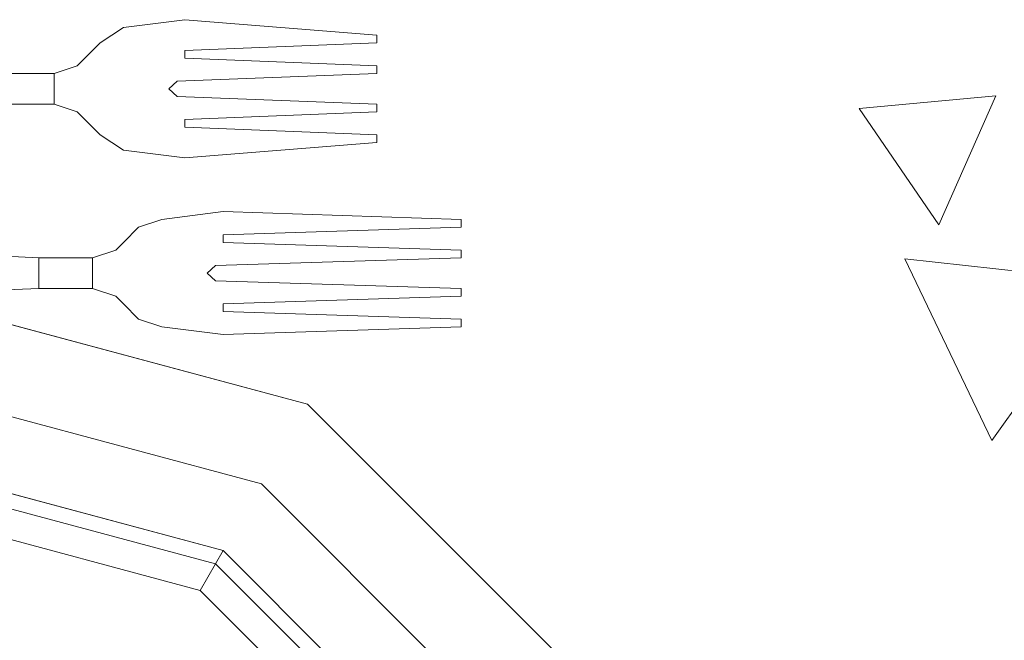
# Model space of a CAD drawing. Units: inches. Extents: x 375 to 1122, y 27 to 1069.
# Tile 103 of 155: x 713.015 to 720.91, y 872.174 to 877.148. Entities that reach past the tile are written whole.
import ezdxf

# ---------------------------------------------------------------- set-up
doc = ezdxf.new("R2010")
doc.units = ezdxf.units.IN
doc.layers.add('Furniture', color=30, linetype='Continuous', lineweight=18)

# ---------------------------------------------------------------- blocks, each defined once
blk = doc.blocks.new('A$C403C54AD')
for p, q in [((1.57741, 0.87913, -0.0006), (1.58183, 0.91926, -0.0006)), ((1.58183, 0.91926, -0.0006), (1.61385, 0.89659, -0.0006)), ((1.54732, 0.87, -0.0006), (1.54475, 0.89734, -0.0006)), ((1.54475, 0.89734, -0.0006), (1.57064, 0.88596, -0.0006)), ((1.61385, 0.89659, -0.0006), (1.57741, 0.87913, -0.0006)), ((1.57064, 0.88596, -0.0006), (1.54732, 0.87, -0.0006)), ((1.56951, 0.73013, -0.02105), (1.57105, 0.72551, -0.02059)), ((1.56951, 0.73013, -0.02413), (1.57105, 0.72551, -0.02367)), ((1.53103, 0.72244, -0.02105), (1.53411, 0.71782, -0.02059)), ((1.53103, 0.72244, -0.02413), (1.53411, 0.71782, -0.02367))]:
    blk.add_line(p, q)
at = {"linetype": 'ByBlock'}
for points, invisible_edges in [([(1.65725, 0.81008, -0.00874), (1.66648, 0.79408, -0.00874), (1.62254, 0.75014, -0.00874), (1.60654, 0.75938, -0.00874)], 5), ([(1.67418, 0.78075, -0.02259), (1.65725, 0.81008, -0.01335), (1.60654, 0.75938, -0.01335), (1.63587, 0.74244, -0.02259)], 5), ([(1.66648, 0.79408, -0.00874), (1.67572, 0.77809, -0.01489), (1.63853, 0.74091, -0.01489), (1.62254, 0.75014, -0.00874)], 5), ([(1.6788, 0.77276, -0.03183), (1.67418, 0.78075, -0.02259), (1.63587, 0.74244, -0.02259), (1.64387, 0.73783, -0.03183)], 1), ([(1.67572, 0.77809, -0.01489), (1.72651, 0.69011, -0.01489), (1.72651, 0.69011, -0.01489), (1.63853, 0.74091, -0.01489)], 5), ([(1.60654, 0.75938, -0.00874), (1.62254, 0.75014, -0.00874), (1.60645, 0.69011, -0.00874), (1.58798, 0.69011, -0.00874)], 5), ([(1.63587, 0.74244, -0.02259), (1.60654, 0.75938, -0.01335), (1.58798, 0.69011, -0.01335), (1.62185, 0.69011, -0.02259)], 5), ([(1.62254, 0.75014, -0.00874), (1.63853, 0.74091, -0.01489), (1.62492, 0.69011, -0.01489), (1.60645, 0.69011, -0.00874)], 5), ([(1.63853, 0.74091, -0.01489), (1.72651, 0.69011, -0.01489), (1.72651, 0.69011, -0.01489), (1.62492, 0.69011, -0.01489)], 5)]:
    blk.add_3dface(points, dxfattribs=dict(at, invisible_edges=invisible_edges))
for points in [[(1.65725, 0.81008, -0.01335), (1.65725, 0.81008, -0.00874), (1.60654, 0.75938, -0.00874), (1.60654, 0.75938, -0.01335)], [(1.60654, 0.75938, -0.01335), (1.60654, 0.75938, -0.00874), (1.58798, 0.69011, -0.00874), (1.58798, 0.69011, -0.01335)], [(1.64387, 0.73783, -0.03183), (1.63587, 0.74244, -0.02259), (1.62185, 0.69011, -0.02259), (1.63108, 0.69011, -0.03183)]]:
    blk.add_3dface(points, dxfattribs=at)
for points, invisible_edges in [([(1.57259, 0.74244, -0.02045), (1.56797, 0.74244, -0.02045), (1.56951, 0.79016, -0.01335), (1.57105, 0.79016, -0.01335)], 1), ([(1.57259, 0.74244, -0.02353), (1.56797, 0.74244, -0.02353), (1.56951, 0.79016, -0.01643), (1.57105, 0.79016, -0.01643)], 1), ([(1.57875, 0.74091, -0.0207), (1.57413, 0.74244, -0.02045), (1.57567, 0.79016, -0.01335), (1.57721, 0.79016, -0.01335)], 1), ([(1.57875, 0.74091, -0.02378), (1.57413, 0.74244, -0.02353), (1.57567, 0.79016, -0.01643), (1.57721, 0.79016, -0.01643)], 1), ([(1.58645, 0.74244, -0.02045), (1.58183, 0.74091, -0.0207), (1.58337, 0.79016, -0.01335), (1.58491, 0.79016, -0.01335)], 1), ([(1.58645, 0.74244, -0.02353), (1.58183, 0.74091, -0.02378), (1.58337, 0.79016, -0.01643), (1.58491, 0.79016, -0.01643)], 1), ([(1.58798, 0.74244, -0.02045), (1.5926, 0.74244, -0.02045), (1.59106, 0.79016, -0.01335), (1.58952, 0.79016, -0.01335)], 1), ([(1.58798, 0.74244, -0.02353), (1.5926, 0.74244, -0.02353), (1.59106, 0.79016, -0.01643), (1.58952, 0.79016, -0.01643)], 1), ([(1.53565, 0.73475, -0.02045), (1.5295, 0.73475, -0.02045), (1.53257, 0.77323, -0.01335), (1.53411, 0.77323, -0.01335)], 1), ([(1.53565, 0.73475, -0.02353), (1.5295, 0.73475, -0.02353), (1.53257, 0.77323, -0.01643), (1.53411, 0.77323, -0.01643)], 1), ([(1.54181, 0.73321, -0.0207), (1.53719, 0.73475, -0.02045), (1.53873, 0.77323, -0.01335), (1.54027, 0.77323, -0.01335)], 1), ([(1.54181, 0.73321, -0.02378), (1.53719, 0.73475, -0.02353), (1.53873, 0.77323, -0.01643), (1.54027, 0.77323, -0.01643)], 1), ([(1.5495, 0.73475, -0.02045), (1.54489, 0.73321, -0.0207), (1.54643, 0.77323, -0.01335), (1.54797, 0.77323, -0.01335)], 1), ([(1.5495, 0.73475, -0.02353), (1.54489, 0.73321, -0.02378), (1.54643, 0.77323, -0.01643), (1.54797, 0.77323, -0.01643)], 1), ([(1.55104, 0.73475, -0.02045), (1.5572, 0.73475, -0.02045), (1.55412, 0.77323, -0.01335), (1.55258, 0.77323, -0.01335)], 1), ([(1.55104, 0.73475, -0.02353), (1.5572, 0.73475, -0.02353), (1.55412, 0.77323, -0.01643), (1.55258, 0.77323, -0.01643)], 1), ([(1.56951, 0.73013, -0.02105), (1.57413, 0.74244, -0.02045), (1.57259, 0.74244, -0.02045), (1.56797, 0.74244, -0.02045)], 5), ([(1.56951, 0.73013, -0.02413), (1.57413, 0.74244, -0.02353), (1.57259, 0.74244, -0.02353), (1.56797, 0.74244, -0.02353)], 5), ([(1.56951, 0.73013, -0.02413), (1.56951, 0.73013, -0.02105), (1.56797, 0.74244, -0.02045), (1.56797, 0.74244, -0.02353)], 1), ([(1.56951, 0.73013, -0.02105), (1.58029, 0.73924, -0.02085), (1.57875, 0.74091, -0.0207), (1.57413, 0.74244, -0.02045)], 13), ([(1.56951, 0.73013, -0.02413), (1.58029, 0.73924, -0.02392), (1.57875, 0.74091, -0.02378), (1.57413, 0.74244, -0.02353)], 13), ([(1.59106, 0.73013, -0.02105), (1.58029, 0.73924, -0.02085), (1.58183, 0.74091, -0.0207), (1.58645, 0.74244, -0.02045)], 13), ([(1.59106, 0.73013, -0.02413), (1.58029, 0.73924, -0.02392), (1.58183, 0.74091, -0.02378), (1.58645, 0.74244, -0.02353)], 13), ([(1.59106, 0.73013, -0.02105), (1.58645, 0.74244, -0.02045), (1.58798, 0.74244, -0.02045), (1.5926, 0.74244, -0.02045)], 5), ([(1.59106, 0.73013, -0.02413), (1.58645, 0.74244, -0.02353), (1.58798, 0.74244, -0.02353), (1.5926, 0.74244, -0.02353)], 5), ([(1.59106, 0.73013, -0.02105), (1.59106, 0.73013, -0.02413), (1.5926, 0.74244, -0.02353), (1.5926, 0.74244, -0.02045)], 1), ([(1.59106, 0.73013, -0.02105), (1.58029, 0.73924, -0.02085), (1.56951, 0.73013, -0.02105), (1.59106, 0.73013, -0.02105)], 7), ([(1.59106, 0.73013, -0.02413), (1.58029, 0.73924, -0.02392), (1.56951, 0.73013, -0.02413), (1.59106, 0.73013, -0.02413)], 7), ([(1.53103, 0.72244, -0.02105), (1.53719, 0.73475, -0.02045), (1.53565, 0.73475, -0.02045), (1.5295, 0.73475, -0.02045)], 5), ([(1.53103, 0.72244, -0.02413), (1.53719, 0.73475, -0.02353), (1.53565, 0.73475, -0.02353), (1.5295, 0.73475, -0.02353)], 5), ([(1.53103, 0.72244, -0.02413), (1.53103, 0.72244, -0.02105), (1.5295, 0.73475, -0.02045), (1.5295, 0.73475, -0.02353)], 1), ([(1.53103, 0.72244, -0.02105), (1.54335, 0.73155, -0.02085), (1.54181, 0.73321, -0.0207), (1.53719, 0.73475, -0.02045)], 13), ([(1.53103, 0.72244, -0.02413), (1.54335, 0.73155, -0.02392), (1.54181, 0.73321, -0.02378), (1.53719, 0.73475, -0.02353)], 13), ([(1.55566, 0.72244, -0.02105), (1.54335, 0.73155, -0.02085), (1.54489, 0.73321, -0.0207), (1.5495, 0.73475, -0.02045)], 13), ([(1.55566, 0.72244, -0.02413), (1.54335, 0.73155, -0.02392), (1.54489, 0.73321, -0.02378), (1.5495, 0.73475, -0.02353)], 13), ([(1.55566, 0.72244, -0.02105), (1.5495, 0.73475, -0.02045), (1.55104, 0.73475, -0.02045), (1.5572, 0.73475, -0.02045)], 5), ([(1.55566, 0.72244, -0.02413), (1.5495, 0.73475, -0.02353), (1.55104, 0.73475, -0.02353), (1.5572, 0.73475, -0.02353)], 5), ([(1.55566, 0.72244, -0.02105), (1.55566, 0.72244, -0.02413), (1.5572, 0.73475, -0.02353), (1.5572, 0.73475, -0.02045)], 1), ([(1.55566, 0.72244, -0.02105), (1.54335, 0.73155, -0.02085), (1.53103, 0.72244, -0.02105), (1.55566, 0.72244, -0.02105)], 7), ([(1.55566, 0.72244, -0.02413), (1.54335, 0.73155, -0.02392), (1.53103, 0.72244, -0.02413), (1.55566, 0.72244, -0.02413)], 7), ([(1.58952, 0.72551, -0.02059), (1.57105, 0.72551, -0.02059), (1.56951, 0.73013, -0.02105), (1.59106, 0.73013, -0.02105)], 5), ([(1.58952, 0.72551, -0.02367), (1.57105, 0.72551, -0.02367), (1.56951, 0.73013, -0.02413), (1.59106, 0.73013, -0.02413)], 5), ([(1.57105, 0.72551, -0.02059), (1.57105, 0.72551, -0.02367), (1.56951, 0.73013, -0.02413), (1.56951, 0.73013, -0.02105)], 4), ([(1.58952, 0.72551, -0.02367), (1.58952, 0.72551, -0.02059), (1.59106, 0.73013, -0.02105), (1.59106, 0.73013, -0.02413)], 4), ([(1.57413, 0.72244, -0.02243), (1.58645, 0.72244, -0.02243), (1.58952, 0.72551, -0.02367), (1.57105, 0.72551, -0.02367)], 5), ([(1.57413, 0.72244, -0.01935), (1.58645, 0.72244, -0.01935), (1.58952, 0.72551, -0.02059), (1.57105, 0.72551, -0.02059)], 5), ([(1.55258, 0.71782, -0.02059), (1.53411, 0.71782, -0.02059), (1.53103, 0.72244, -0.02105), (1.55566, 0.72244, -0.02105)], 5), ([(1.55258, 0.71782, -0.02367), (1.53411, 0.71782, -0.02367), (1.53103, 0.72244, -0.02413), (1.55566, 0.72244, -0.02413)], 5), ([(1.53411, 0.71782, -0.02059), (1.53411, 0.71782, -0.02367), (1.53103, 0.72244, -0.02413), (1.53103, 0.72244, -0.02105)], 4), ([(1.55258, 0.71782, -0.02367), (1.55258, 0.71782, -0.02059), (1.55566, 0.72244, -0.02105), (1.55566, 0.72244, -0.02413)], 4), ([(1.57567, 0.7209, -0.0183), (1.58491, 0.7209, -0.0183), (1.58645, 0.72244, -0.01935), (1.57413, 0.72244, -0.01935)], 5), ([(1.57567, 0.7209, -0.02109), (1.58491, 0.7209, -0.02109), (1.58645, 0.72244, -0.02243), (1.57413, 0.72244, -0.02243)], 5), ([(1.57567, 0.7209, -0.0183), (1.57567, 0.7209, -0.02109), (1.57413, 0.72244, -0.02243), (1.57413, 0.72244, -0.01935)], 1), ([(1.58337, 0.71628, -0.01595), (1.57721, 0.71628, -0.01595), (1.57567, 0.7209, -0.0183), (1.58491, 0.7209, -0.0183)], 4), ([(1.57721, 0.71628, -0.01854), (1.57721, 0.71628, -0.01595), (1.57567, 0.7209, -0.0183), (1.57567, 0.7209, -0.02109)], 5), ([(1.58337, 0.71628, -0.01854), (1.57721, 0.71628, -0.01854), (1.57567, 0.7209, -0.02109), (1.58491, 0.7209, -0.02109)], 4), ([(1.58337, 0.71628, -0.01595), (1.58337, 0.71628, -0.01854), (1.58491, 0.7209, -0.02109), (1.58491, 0.7209, -0.0183)], 5), ([(1.58491, 0.7209, -0.02109), (1.58491, 0.7209, -0.0183), (1.58645, 0.72244, -0.01935), (1.58645, 0.72244, -0.02243)], 1), ([(1.53719, 0.71474, -0.02243), (1.5495, 0.71474, -0.02243), (1.55258, 0.71782, -0.02367), (1.53411, 0.71782, -0.02367)], 5), ([(1.53719, 0.71474, -0.01935), (1.5495, 0.71474, -0.01935), (1.55258, 0.71782, -0.02059), (1.53411, 0.71782, -0.02059)], 5), ([(1.53873, 0.7132, -0.0183), (1.54797, 0.7132, -0.0183), (1.5495, 0.71474, -0.01935), (1.53719, 0.71474, -0.01935)], 5), ([(1.53873, 0.7132, -0.02109), (1.54797, 0.7132, -0.02109), (1.5495, 0.71474, -0.02243), (1.53719, 0.71474, -0.02243)], 5), ([(1.53873, 0.7132, -0.0183), (1.53873, 0.7132, -0.02109), (1.53719, 0.71474, -0.02243), (1.53719, 0.71474, -0.01935)], 1), ([(1.54797, 0.7132, -0.02109), (1.54797, 0.7132, -0.0183), (1.5495, 0.71474, -0.01935), (1.5495, 0.71474, -0.02243)], 1), ([(1.57721, 0.71628, -0.01854), (1.57721, 0.71628, -0.01595), (1.57721, 0.7055, -0.01387), (1.57721, 0.7055, -0.01646)], 5), ([(1.58337, 0.7055, -0.01646), (1.58337, 0.7055, -0.01387), (1.58337, 0.71628, -0.01595), (1.58337, 0.71628, -0.01854)], 5), ([(1.54643, 0.70858, -0.01595), (1.54027, 0.70858, -0.01595), (1.53873, 0.7132, -0.0183), (1.54797, 0.7132, -0.0183)], 4), ([(1.54643, 0.70858, -0.01854), (1.54027, 0.70858, -0.01854), (1.53873, 0.7132, -0.02109), (1.54797, 0.7132, -0.02109)], 4), ([(1.54027, 0.70858, -0.01854), (1.54027, 0.70858, -0.01595), (1.53873, 0.7132, -0.0183), (1.53873, 0.7132, -0.02109)], 5), ([(1.54643, 0.70858, -0.01595), (1.54643, 0.70858, -0.01854), (1.54797, 0.7132, -0.02109), (1.54797, 0.7132, -0.0183)], 5), ([(1.54027, 0.70858, -0.01854), (1.54027, 0.70858, -0.01595), (1.54027, 0.69781, -0.01387), (1.54027, 0.69781, -0.01646)], 5), ([(1.54643, 0.69781, -0.01646), (1.54643, 0.69781, -0.01387), (1.54643, 0.70858, -0.01595), (1.54643, 0.70858, -0.01854)], 5), ([(1.58491, 0.6701, -0.01678), (1.57567, 0.6701, -0.01678), (1.57721, 0.7055, -0.01387), (1.58337, 0.7055, -0.01387)], 1), ([(1.57721, 0.7055, -0.01387), (1.57721, 0.7055, -0.01646), (1.57567, 0.6701, -0.01986), (1.57567, 0.6701, -0.01678)], 5), ([(1.58491, 0.6701, -0.01986), (1.57567, 0.6701, -0.01986), (1.57721, 0.7055, -0.01646), (1.58337, 0.7055, -0.01646)], 1), ([(1.58491, 0.6701, -0.01678), (1.58491, 0.6701, -0.01986), (1.58337, 0.7055, -0.01646), (1.58337, 0.7055, -0.01387)], 5)]:
    blk.add_3dface(points, dxfattribs=dict(invisible_edges=invisible_edges))
for points in [[(1.56951, 0.79016, -0.01335), (1.56951, 0.79016, -0.01643), (1.56797, 0.74244, -0.02353), (1.56797, 0.74244, -0.02045)], [(1.57105, 0.79016, -0.01643), (1.57105, 0.79016, -0.01335), (1.56951, 0.79016, -0.01335), (1.56951, 0.79016, -0.01643)], [(1.57259, 0.74244, -0.02045), (1.57259, 0.74244, -0.02353), (1.57105, 0.79016, -0.01643), (1.57105, 0.79016, -0.01335)], [(1.57567, 0.79016, -0.01335), (1.57567, 0.79016, -0.01643), (1.57413, 0.74244, -0.02353), (1.57413, 0.74244, -0.02045)], [(1.57721, 0.79016, -0.01643), (1.57721, 0.79016, -0.01335), (1.57567, 0.79016, -0.01335), (1.57567, 0.79016, -0.01643)], [(1.57875, 0.74091, -0.02378), (1.57875, 0.74091, -0.0207), (1.57721, 0.79016, -0.01335), (1.57721, 0.79016, -0.01643)], [(1.58337, 0.79016, -0.01643), (1.58337, 0.79016, -0.01335), (1.58183, 0.74091, -0.0207), (1.58183, 0.74091, -0.02378)], [(1.58491, 0.79016, -0.01643), (1.58491, 0.79016, -0.01335), (1.58337, 0.79016, -0.01335), (1.58337, 0.79016, -0.01643)], [(1.58645, 0.74244, -0.02353), (1.58645, 0.74244, -0.02045), (1.58491, 0.79016, -0.01335), (1.58491, 0.79016, -0.01643)], [(1.58952, 0.79016, -0.01335), (1.58952, 0.79016, -0.01643), (1.58798, 0.74244, -0.02353), (1.58798, 0.74244, -0.02045)], [(1.59106, 0.79016, -0.01643), (1.59106, 0.79016, -0.01335), (1.58952, 0.79016, -0.01335), (1.58952, 0.79016, -0.01643)], [(1.5926, 0.74244, -0.02353), (1.5926, 0.74244, -0.02045), (1.59106, 0.79016, -0.01335), (1.59106, 0.79016, -0.01643)], [(1.53257, 0.77323, -0.01335), (1.53257, 0.77323, -0.01643), (1.5295, 0.73475, -0.02353), (1.5295, 0.73475, -0.02045)], [(1.53411, 0.77323, -0.01643), (1.53411, 0.77323, -0.01335), (1.53257, 0.77323, -0.01335), (1.53257, 0.77323, -0.01643)], [(1.53565, 0.73475, -0.02045), (1.53565, 0.73475, -0.02353), (1.53411, 0.77323, -0.01643), (1.53411, 0.77323, -0.01335)], [(1.53873, 0.77323, -0.01335), (1.53873, 0.77323, -0.01643), (1.53719, 0.73475, -0.02353), (1.53719, 0.73475, -0.02045)], [(1.54027, 0.77323, -0.01643), (1.54027, 0.77323, -0.01335), (1.53873, 0.77323, -0.01335), (1.53873, 0.77323, -0.01643)], [(1.54181, 0.73321, -0.02378), (1.54181, 0.73321, -0.0207), (1.54027, 0.77323, -0.01335), (1.54027, 0.77323, -0.01643)], [(1.54643, 0.77323, -0.01643), (1.54643, 0.77323, -0.01335), (1.54489, 0.73321, -0.0207), (1.54489, 0.73321, -0.02378)], [(1.54797, 0.77323, -0.01643), (1.54797, 0.77323, -0.01335), (1.54643, 0.77323, -0.01335), (1.54643, 0.77323, -0.01643)], [(1.5495, 0.73475, -0.02353), (1.5495, 0.73475, -0.02045), (1.54797, 0.77323, -0.01335), (1.54797, 0.77323, -0.01643)], [(1.55258, 0.77323, -0.01335), (1.55258, 0.77323, -0.01643), (1.55104, 0.73475, -0.02353), (1.55104, 0.73475, -0.02045)], [(1.55412, 0.77323, -0.01643), (1.55412, 0.77323, -0.01335), (1.55258, 0.77323, -0.01335), (1.55258, 0.77323, -0.01643)], [(1.5572, 0.73475, -0.02353), (1.5572, 0.73475, -0.02045), (1.55412, 0.77323, -0.01335), (1.55412, 0.77323, -0.01643)], [(1.57259, 0.74244, -0.02045), (1.57259, 0.74244, -0.02353), (1.57413, 0.74244, -0.02353), (1.57413, 0.74244, -0.02045)], [(1.58645, 0.74244, -0.02353), (1.58645, 0.74244, -0.02045), (1.58798, 0.74244, -0.02045), (1.58798, 0.74244, -0.02353)], [(1.57875, 0.74091, -0.0207), (1.57875, 0.74091, -0.02378), (1.58029, 0.73924, -0.02392), (1.58029, 0.73924, -0.02085)], [(1.58029, 0.73924, -0.02392), (1.58029, 0.73924, -0.02085), (1.58183, 0.74091, -0.0207), (1.58183, 0.74091, -0.02378)], [(1.53565, 0.73475, -0.02045), (1.53565, 0.73475, -0.02353), (1.53719, 0.73475, -0.02353), (1.53719, 0.73475, -0.02045)], [(1.5495, 0.73475, -0.02353), (1.5495, 0.73475, -0.02045), (1.55104, 0.73475, -0.02045), (1.55104, 0.73475, -0.02353)], [(1.54181, 0.73321, -0.0207), (1.54181, 0.73321, -0.02378), (1.54335, 0.73155, -0.02392), (1.54335, 0.73155, -0.02085)], [(1.54335, 0.73155, -0.02392), (1.54335, 0.73155, -0.02085), (1.54489, 0.73321, -0.0207), (1.54489, 0.73321, -0.02378)], [(1.57413, 0.72244, -0.02243), (1.57413, 0.72244, -0.01935), (1.57105, 0.72551, -0.02059), (1.57105, 0.72551, -0.02367)], [(1.58645, 0.72244, -0.01935), (1.58645, 0.72244, -0.02243), (1.58952, 0.72551, -0.02367), (1.58952, 0.72551, -0.02059)], [(1.53719, 0.71474, -0.02243), (1.53719, 0.71474, -0.01935), (1.53411, 0.71782, -0.02059), (1.53411, 0.71782, -0.02367)], [(1.5495, 0.71474, -0.01935), (1.5495, 0.71474, -0.02243), (1.55258, 0.71782, -0.02367), (1.55258, 0.71782, -0.02059)], [(1.57721, 0.7055, -0.01387), (1.58337, 0.7055, -0.01387), (1.58337, 0.71628, -0.01595), (1.57721, 0.71628, -0.01595)], [(1.57721, 0.7055, -0.01646), (1.58337, 0.7055, -0.01646), (1.58337, 0.71628, -0.01854), (1.57721, 0.71628, -0.01854)], [(1.54027, 0.69781, -0.01387), (1.54643, 0.69781, -0.01387), (1.54643, 0.70858, -0.01595), (1.54027, 0.70858, -0.01595)], [(1.54027, 0.69781, -0.01646), (1.54643, 0.69781, -0.01646), (1.54643, 0.70858, -0.01854), (1.54027, 0.70858, -0.01854)]]:
    blk.add_3dface(points)

msp = doc.modelspace()

# ---------------------------------------------------------------- block references
at = {"layer": 'Furniture', "xscale": 39.9918517141215, "yscale": 39.9918517141215, "zscale": 39.9918517141215, "rotation": 270}
msp.add_blockref('A$C403C54AD', (684.9549, 938.3156, 0.024), dxfattribs=at)

doc.saveas('drawing.dxf')
